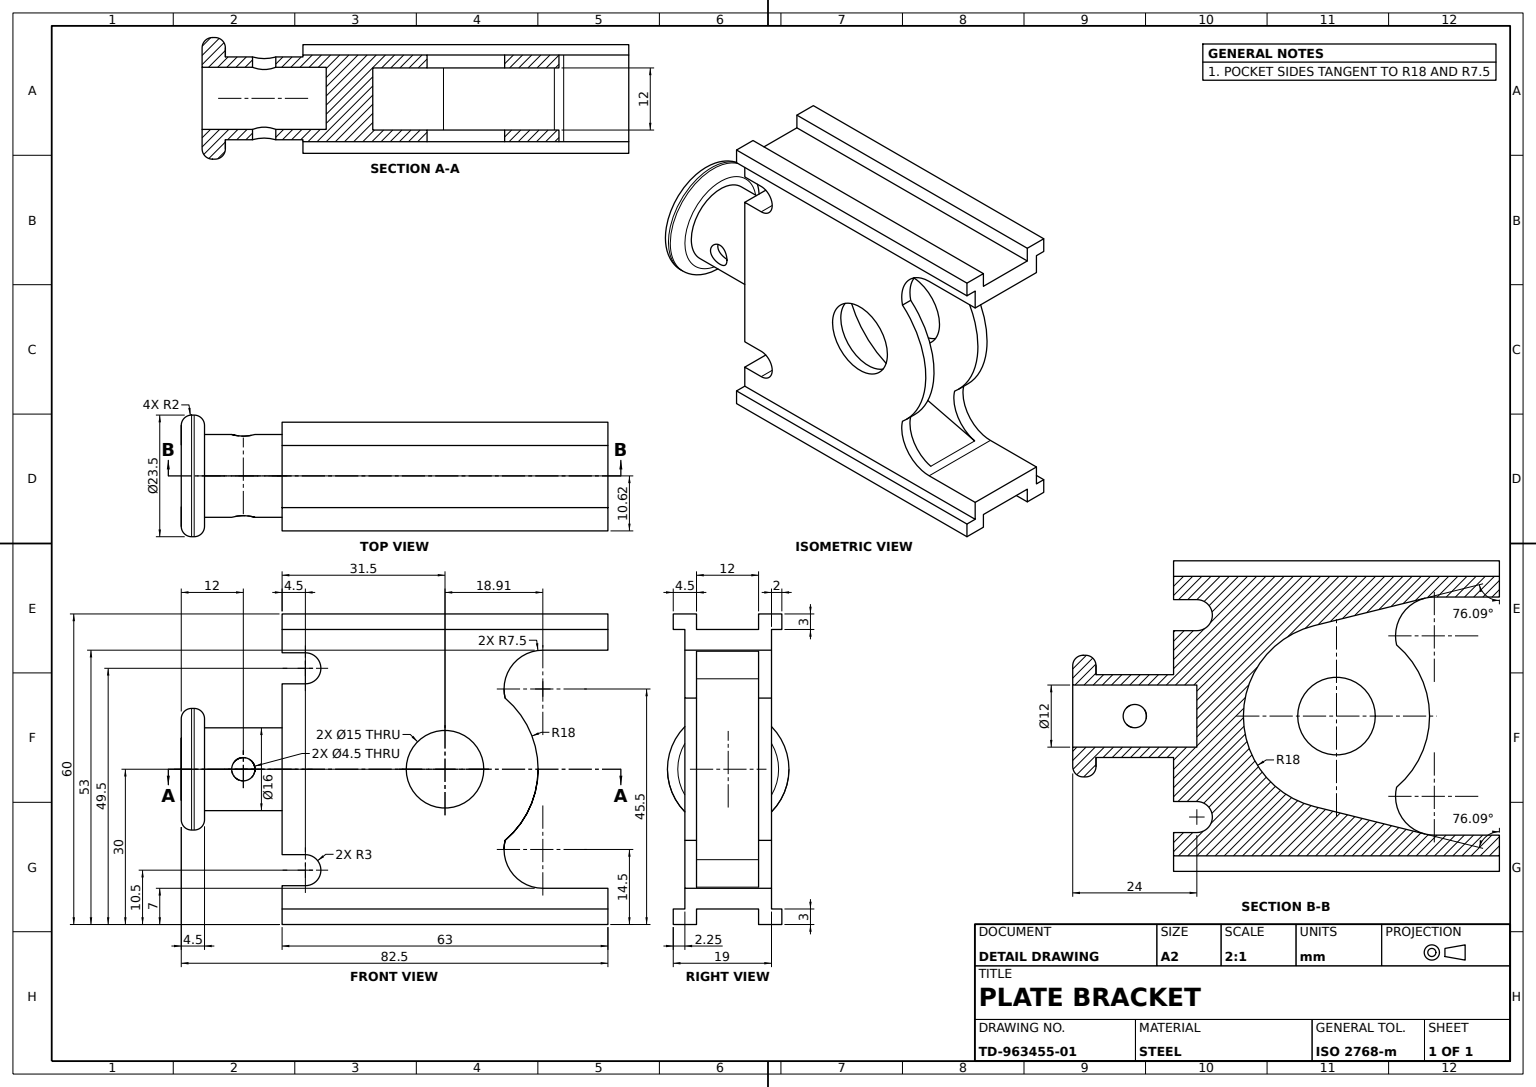
from build123d import *

# Parameters (mm, degrees)
I_SECTION_PROFILE_SKETCH_W   = 63
I_SECTION_PROFILE_SKETCH_H   = 3
I_SECTION_PROFILE_SKETCH_R   = 18
I_SECTION_PROFILE_SKETCH_R_2 = 7.5
BASE_PLATE_2_25_DEPTH        = 2.25
SKETCH1_11_W                 = 63
SKETCH1_11_H                 = 3
SECTION_STEP_4_5_DEPTH       = 4.5
SECTION_STEP_12_DEPTH        = 12
SECTION_START                = -14.5
SKETCH1_14_W                 = 63
SKETCH1_14_H                 = 3
SKETCH1_14_R                 = 18
SKETCH1_14_R_2               = 7.5
SECTION_STEP_2_5_DEPTH       = 2.5
SECTION_START_2              = -12
SECTION_STEP_TO_FACE_DEPTH   = 12
SKETCH1_16_W                 = 63
SKETCH1_16_H                 = 3
SECTION_STEP_2_DEPTH         = 2
HUB_SKETCH_16_R              = 8
HUB_16_DEPTH                 = 19.5
FLANGE_SKETCH_23_5_R         = 11.75
FLANGE_23_5_DEPTH            = 4.5
BORE_SKETCH_12_R             = 6
BORE_12_DEPTH                = 24
CROSS_HOLE_4_5_DEPTH         = 62.810319729
CROSS_HOLE_4_5_DEPTH_BACK    = 62.810319729
CROSS_HOLE_SKETCH_4_5_R      = 2.25
FLANGE_FILLET_R2_R           = 2


with BuildPart() as part:
    # I-Section Profile Sketch → Base Plate 2.25 (new body)
    # profile 1 of 8: a face of its own
    with BuildSketch(Plane.XY):
        with Locations((0, 28.5)):
            Rectangle(I_SECTION_PROFILE_SKETCH_W, I_SECTION_PROFILE_SKETCH_H)
    # profile 2 of 8: a face of its own
    with BuildSketch(Plane.XY):
        Polygon((-31.5, 27), (-31.5, 23), (18.914634146, 23), (31.5, 23), (31.5, 27), align=None)
    # profile 3 of 8: a face of its own
    with BuildSketch(Plane.XY):
        with BuildLine():
            ThreePointArc((11.623034417, 13.744274115), (12.504687014, 19.39391548), (17.112172247, 22.780187573))
            Line((17.112172247, 22.780187573), (-4.325908558, 17.472450176))
            ThreePointArc((-4.325908558, 17.472450176), (4.097174104, 17.527497379), (11.623034417, 13.744274115))
        make_face()
    # profile 4 of 8: a face of its own
    with BuildSketch(Plane.XY):
        with BuildLine():
            Line((-31.5, 22.5), (-27, 22.5))
            ThreePointArc((-27, 22.5), (-24, 19.5), (-27, 16.5))
            Line((-27, 16.5), (-31.5, 16.5))
            Line((-31.5, 16.5), (-31.5, -16.5))
            Line((-31.5, -16.5), (-27, -16.5))
            ThreePointArc((-27, -16.5), (-24, -19.5), (-27, -22.5))
            Line((-27, -22.5), (-31.5, -22.5))
            Line((-31.5, -22.5), (-31.5, -23))
            Line((-31.5, -23), (18.914634146, -23))
            ThreePointArc((18.914634146, -23), (18.006726332, -22.944844082), (17.112172247, -22.780187573))
            Line((17.112172247, -22.780187573), (-4.325908558, -17.472450176))
            ThreePointArc((-4.325908558, -17.472450176), (-18, 0), (-4.325908558, 17.472450176))
            Line((-4.325908558, 17.472450176), (17.112172247, 22.780187573))
            ThreePointArc((17.112172247, 22.780187573), (18.006726332, 22.944844082), (18.914634146, 23))
            Line((18.914634146, 23), (-31.5, 23))
            Line((-31.5, 23), (-31.5, 22.5))
        make_face()
    # profile 5 of 8: a face of its own
    with BuildSketch(Plane.XY):
        Circle(I_SECTION_PROFILE_SKETCH_R)
        Circle(I_SECTION_PROFILE_SKETCH_R_2, mode=Mode.SUBTRACT)
    # profile 6 of 8: a face of its own
    with BuildSketch(Plane.XY):
        Polygon((31.5, -27), (31.5, -23), (18.914634146, -23), (-31.5, -23), (-31.5, -27), align=None)
    # profile 7 of 8: a face of its own
    with BuildSketch(Plane.XY):
        with Locations((0, -28.5)):
            Rectangle(I_SECTION_PROFILE_SKETCH_W, I_SECTION_PROFILE_SKETCH_H)
    # profile 8 of 8: a face of its own
    with BuildSketch(Plane.XY):
        with BuildLine():
            ThreePointArc((11.623034417, -13.744274115), (4.097174104, -17.527497379), (-4.325908558, -17.472450176))
            Line((-4.325908558, -17.472450176), (17.112172247, -22.780187573))
            ThreePointArc((17.112172247, -22.780187573), (12.504687014, -19.39391548), (11.623034417, -13.744274115))
        make_face()
    extrude(amount=BASE_PLATE_2_25_DEPTH)

    # Sketch1_11 → Section Step 4.5 (add)
    with BuildSketch(Plane.XY):
        with Locations((0, 28.5)):
            Rectangle(SKETCH1_11_W, SKETCH1_11_H)
        with Locations((0, -28.5)):
            Rectangle(SKETCH1_11_W, SKETCH1_11_H)
    extrude(amount=SECTION_STEP_4_5_DEPTH)

    # Sketch1_13 → Section Step 12 (add)
    with BuildSketch(Plane.XY):
        Polygon((-31.5, 27), (-31.5, 23), (18.914634146, 23), (31.5, 23), (31.5, 27), align=None)
        Polygon((31.5, -27), (31.5, -23), (18.914634146, -23), (-31.5, -23), (-31.5, -27), align=None)
    extrude(amount=-SECTION_STEP_12_DEPTH)

    # Sketch1_14 → Section Step 2.5 (add)
    # profile 1 of 8: a face of its own
    with BuildSketch(Plane.XY.offset(SECTION_START)):
        with Locations((0, 28.5)):
            Rectangle(SKETCH1_14_W, SKETCH1_14_H)
    # profile 2 of 8: a face of its own
    with BuildSketch(Plane.XY.offset(SECTION_START)):
        Polygon((-31.5, 27), (-31.5, 23), (18.914634146, 23), (31.5, 23), (31.5, 27), align=None)
    # profile 3 of 8: a face of its own
    with BuildSketch(Plane.XY.offset(SECTION_START)):
        with BuildLine():
            Line((-31.5, 22.5), (-27, 22.5))
            ThreePointArc((-27, 22.5), (-24, 19.5), (-27, 16.5))
            Line((-27, 16.5), (-31.5, 16.5))
            Line((-31.5, 16.5), (-31.5, -16.5))
            Line((-31.5, -16.5), (-27, -16.5))
            ThreePointArc((-27, -16.5), (-24, -19.5), (-27, -22.5))
            Line((-27, -22.5), (-31.5, -22.5))
            Line((-31.5, -22.5), (-31.5, -23))
            Line((-31.5, -23), (18.914634146, -23))
            ThreePointArc((18.914634146, -23), (18.006726332, -22.944844082), (17.112172247, -22.780187573))
            Line((17.112172247, -22.780187573), (-4.325908558, -17.472450176))
            ThreePointArc((-4.325908558, -17.472450176), (-18, 0), (-4.325908558, 17.472450176))
            Line((-4.325908558, 17.472450176), (17.112172247, 22.780187573))
            ThreePointArc((17.112172247, 22.780187573), (18.006726332, 22.944844082), (18.914634146, 23))
            Line((18.914634146, 23), (-31.5, 23))
            Line((-31.5, 23), (-31.5, 22.5))
        make_face()
    # profile 4 of 8: a face of its own
    with BuildSketch(Plane.XY.offset(SECTION_START)):
        Circle(SKETCH1_14_R)
        Circle(SKETCH1_14_R_2, mode=Mode.SUBTRACT)
    # profile 5 of 8: a face of its own
    with BuildSketch(Plane.XY.offset(SECTION_START)):
        with BuildLine():
            ThreePointArc((11.623034417, 13.744274115), (12.504687014, 19.39391548), (17.112172247, 22.780187573))
            Line((17.112172247, 22.780187573), (-4.325908558, 17.472450176))
            ThreePointArc((-4.325908558, 17.472450176), (4.097174104, 17.527497379), (11.623034417, 13.744274115))
        make_face()
    # profile 6 of 8: a face of its own
    with BuildSketch(Plane.XY.offset(SECTION_START)):
        with BuildLine():
            ThreePointArc((11.623034417, -13.744274115), (4.097174104, -17.527497379), (-4.325908558, -17.472450176))
            Line((-4.325908558, -17.472450176), (17.112172247, -22.780187573))
            ThreePointArc((17.112172247, -22.780187573), (12.504687014, -19.39391548), (11.623034417, -13.744274115))
        make_face()
    # profile 7 of 8: a face of its own
    with BuildSketch(Plane.XY.offset(SECTION_START)):
        Polygon((31.5, -27), (31.5, -23), (18.914634146, -23), (-31.5, -23), (-31.5, -27), align=None)
    # profile 8 of 8: a face of its own
    with BuildSketch(Plane.XY.offset(SECTION_START)):
        with Locations((0, -28.5)):
            Rectangle(SKETCH1_14_W, SKETCH1_14_H)
    extrude(amount=SECTION_STEP_2_5_DEPTH)

    # Sketch1_15 → Section Step To Face (add)
    with BuildSketch(Plane.XY.offset(SECTION_START_2)):
        with BuildLine():
            Line((-31.5, 22.5), (-27, 22.5))
            ThreePointArc((-27, 22.5), (-24, 19.5), (-27, 16.5))
            Line((-27, 16.5), (-31.5, 16.5))
            Line((-31.5, 16.5), (-31.5, -16.5))
            Line((-31.5, -16.5), (-27, -16.5))
            ThreePointArc((-27, -16.5), (-24, -19.5), (-27, -22.5))
            Line((-27, -22.5), (-31.5, -22.5))
            Line((-31.5, -22.5), (-31.5, -23))
            Line((-31.5, -23), (18.914634146, -23))
            ThreePointArc((18.914634146, -23), (18.006726332, -22.944844082), (17.112172247, -22.780187573))
            Line((17.112172247, -22.780187573), (-4.325908558, -17.472450176))
            ThreePointArc((-4.325908558, -17.472450176), (-18, 0), (-4.325908558, 17.472450176))
            Line((-4.325908558, 17.472450176), (17.112172247, 22.780187573))
            ThreePointArc((17.112172247, 22.780187573), (18.006726332, 22.944844082), (18.914634146, 23))
            Line((18.914634146, 23), (-31.5, 23))
            Line((-31.5, 23), (-31.5, 22.5))
        make_face()
    extrude(amount=SECTION_STEP_TO_FACE_DEPTH)

    # Sketch1_16 → Section Step 2 (add)
    with BuildSketch(Plane.XY.offset(SECTION_START)):
        with Locations((0, 28.5)):
            Rectangle(SKETCH1_16_W, SKETCH1_16_H)
        with Locations((0, -28.5)):
            Rectangle(SKETCH1_16_W, SKETCH1_16_H)
    extrude(amount=-SECTION_STEP_2_DEPTH)

    # Hub Sketch _16 → Hub _16 (add)
    with BuildSketch(Plane.ZY.offset(31.5)):
        with Locations((-6.125, 0)):
            Circle(HUB_SKETCH_16_R)
    extrude(amount=HUB_16_DEPTH)

    # Flange Sketch _23.5 → Flange _23.5 (add)
    with BuildSketch(Plane.ZY.offset(51)):
        with Locations((-6.125, 0)):
            Circle(FLANGE_SKETCH_23_5_R)
    extrude(amount=-FLANGE_23_5_DEPTH)

    # Bore Sketch _12 → Bore _12 (cut)
    with BuildSketch(Plane.ZY.offset(51)):
        with Locations((-6.125, 0)):
            Circle(BORE_SKETCH_12_R)
    extrude(amount=-BORE_12_DEPTH, mode=Mode.SUBTRACT)

    # Cross Hole Sketch _4.5 → Cross Hole _4.5 (cut, two sides: drawn at the far end of the back side and taken through both)
    with BuildSketch(Plane.XY.offset(-CROSS_HOLE_4_5_DEPTH_BACK)):
        with Locations((-39, 0)):
            Circle(CROSS_HOLE_SKETCH_4_5_R)
    extrude(amount=CROSS_HOLE_4_5_DEPTH + CROSS_HOLE_4_5_DEPTH_BACK, mode=Mode.SUBTRACT)

    # Flange Fillet R2
    flange_fillet_r2_edges = [part.edges().sort_by_distance(p)[0] for p in [
        (-46.5, 0, -17.875),
        (-51, 0, -17.875),
    ]]
    fillet(flange_fillet_r2_edges, radius=FLANGE_FILLET_R2_R)


solid = part.part
